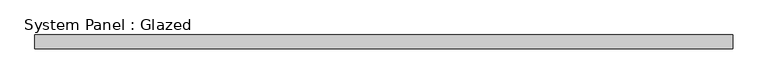
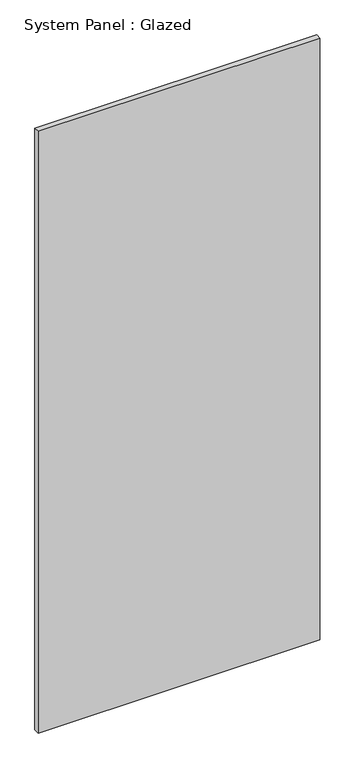
"""IFC4 building model written with IfcOpenShell, lengths in millimetres: plate geometry, System Panel : Glazed."""

from ifc_helpers import new_model, si_unit, origin, origin_with_axes, place, context, project, spatial, polyline, outline, extrude, source, transform, mapped, element, save


def system_panel_glazed_5b6ff290(model_context):
    return source(origin(), model_context, "Body", "SweptSolid", [
        extrude(outline(polyline([(647.2276162, 19.05), (-647.2276162, 19.05), (-647.2276162, 44.45), (647.2276162, 44.45), (647.2276162, 19.05)])), origin_with_axes(), (0.0, 0.0, 1.0), 2921.0),
    ])


if __name__ == "__main__":
    model = new_model("IFC4")
    model_context = context("Model", 3, world=origin())
    ifc_project = project(units=[si_unit("LENGTHUNIT", "METRE", prefix="MILLI")], contexts=[model_context])
    site = spatial("IfcSite", under=ifc_project)
    building = spatial("IfcBuilding", under=site)
    placement = place(None, origin())
    system_panel_glazed_shape = system_panel_glazed_5b6ff290(model_context)
    element("IfcPlate", 1, ObjectType="System Panel : Glazed", at=placement, inside=building, context=model_context, shape_type="MappedRepresentation", body=[
        mapped(system_panel_glazed_shape, transform((0.0, 0.0, 0.0), x_axis=(1.0, 0.0, 0.0), y_axis=(0.0, 1.0, 0.0), z_axis=(0.0, 0.0, 1.0))),
    ])
    save(model, "model.ifc")

# Revit data of these elements
# Type "System Panel : Glazed"
#   Construction Type Id = "GSP4R"
#   Analytic Construction = "1/8 in Pilkington single glazing"
#   Visual Light Transmittance = 0.9
#   Solar Heat Gain Coefficient = 0.86
#   Heat Transfer Coefficient (U) = 1.18115 BTU/(h·ft²·°F)
# Element 1 (IfcPlate, "System Panel : Glazed")
#   Materials on its faces: "Glass"
# Materials
#   "Glass": class "Glass", colour RGB 0 128 192, transparency 0.75, Description = "Soda Lime Glass", Cost = 0
